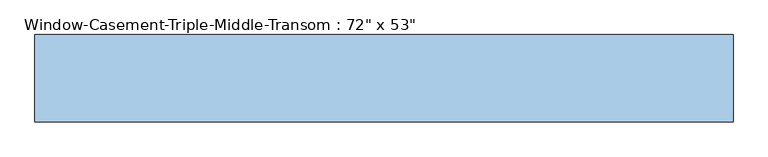
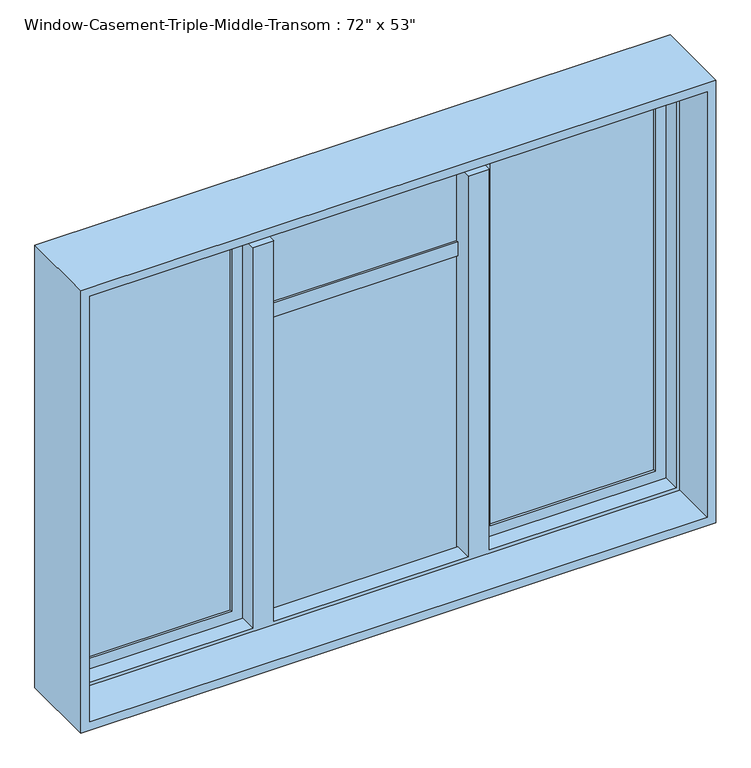
"""IFC4 building model written with IfcOpenShell, lengths in millimetres: window geometry."""

from ifc_helpers import new_model, si_unit, frame, origin, place, context, project, spatial, polyline, outline, extrude, faceted_brep, source, transform, mapped, element, save


def window_7a1f68bc(model_context):
    return source(origin(), model_context, "Body", "SolidModel", [
        extrude(outline(polyline([(2235.2, 330.2), (939.8, 330.2), (939.8, 889.0), (2235.2, 889.0), (2235.2, 330.2)]), holes=[polyline([(2193.3296875, 847.1296875), (981.6703125, 847.1296875), (981.6703125, 372.0703125), (2193.3296875, 372.0703125), (2193.3296875, 847.1296875)])]), frame((0.0, 73.025, 0.0), z_axis=(0.0, 1.0, 0.0), x_axis=(0.0, 0.0, 1.0)), (0.0, 0.0, 1.0), 31.75),
        extrude(outline(polyline([(2235.2, -889.0), (939.8, -889.0), (939.8, -330.2), (2235.2, -330.2), (2235.2, -889.0)]), holes=[polyline([(2193.3296875, -372.0703125), (981.6703125, -372.0703125), (981.6703125, -847.1296875), (2193.3296875, -847.1296875), (2193.3296875, -372.0703125)])]), frame((0.0, 73.025, 0.0), z_axis=(0.0, 1.0, 0.0), x_axis=(0.0, 0.0, 1.0)), (0.0, 0.0, 1.0), 31.75),
        extrude(outline(polyline([(-372.0703125, 98.425), (-372.0703125, 92.075), (-847.1296875, 92.075), (-847.1296875, 98.425), (-372.0703125, 98.425)])), frame((0.0, 0.0, 949.9203125), z_axis=(0.0, 0.0, 1.0), x_axis=(1.0, 0.0, 0.0)), (0.0, 0.0, 1.0), 1275.159375),
        extrude(outline(polyline([(-372.0703125, 85.725), (-372.0703125, 79.375), (-847.1296875, 79.375), (-847.1296875, 85.725), (-372.0703125, 85.725)])), frame((0.0, 0.0, 949.9203125), z_axis=(0.0, 0.0, 1.0), x_axis=(1.0, 0.0, 0.0)), (0.0, 0.0, 1.0), 1275.159375),
        extrude(outline(polyline([(847.1296875, 98.425), (847.1296875, 92.075), (372.0703125, 92.075), (372.0703125, 98.425), (847.1296875, 98.425)])), frame((0.0, 0.0, 949.9203125), z_axis=(0.0, 0.0, 1.0), x_axis=(1.0, 0.0, 0.0)), (0.0, 0.0, 1.0), 1275.159375),
        extrude(outline(polyline([(847.1296875, 85.725), (847.1296875, 79.375), (372.0703125, 79.375), (372.0703125, 85.725), (847.1296875, 85.725)])), frame((0.0, 0.0, 949.9203125), z_axis=(0.0, 0.0, 1.0), x_axis=(1.0, 0.0, 0.0)), (0.0, 0.0, 1.0), 1275.159375),
        extrude(outline(polyline([(279.4, 104.775), (279.4, 73.025), (-279.4, 73.025), (-279.4, 104.775), (279.4, 104.775)])), frame((0.0, 0.0, 1835.8048438), z_axis=(0.0, 0.0, 1.0), x_axis=(1.0, 0.0, 0.0)), (0.0, 0.0, 1.0), 41.8703125),
        extrude(outline(polyline([(279.4, 98.425), (279.4, 92.075), (-279.4, 92.075), (-279.4, 98.425), (279.4, 98.425)])), frame((0.0, 0.0, 939.8), z_axis=(0.0, 0.0, 1.0), x_axis=(1.0, 0.0, 0.0)), (0.0, 0.0, 1.0), 896.0048437),
        extrude(outline(polyline([(279.4, 85.725), (279.4, 79.375), (-279.4, 79.375), (-279.4, 85.725), (279.4, 85.725)])), frame((0.0, 0.0, 939.8), z_axis=(0.0, 0.0, 1.0), x_axis=(1.0, 0.0, 0.0)), (0.0, 0.0, 1.0), 896.0048437),
        extrude(outline(polyline([(279.4, 98.425), (279.4, 92.075), (-279.4, 92.075), (-279.4, 98.425), (279.4, 98.425)])), frame((0.0, 0.0, 1877.6751563), z_axis=(0.0, 0.0, 1.0), x_axis=(1.0, 0.0, 0.0)), (0.0, 0.0, 1.0), 357.5248438),
        extrude(outline(polyline([(279.4, 85.725), (279.4, 79.375), (-279.4, 79.375), (-279.4, 85.725), (279.4, 85.725)])), frame((0.0, 0.0, 1877.6751563), z_axis=(0.0, 0.0, 1.0), x_axis=(1.0, 0.0, 0.0)), (0.0, 0.0, 1.0), 357.5248438),
        faceted_brep([(-889.0, 73.025, 2235.2), (-889.0, 114.3, 2235.2), (889.0, 114.3, 2235.2), (889.0, 73.025, 2235.2), (-878.8796875, 22.225, 2225.0796875), (-878.8796875, 73.025, 2225.0796875), (878.8796875, 73.025, 2225.0796875), (878.8796875, 22.225, 2225.0796875), (-889.0, -114.3, 2235.2), (-889.0, 22.225, 2235.2), (889.0, 22.225, 2235.2), (889.0, -114.3, 2235.2), (-914.4, 114.3, 2260.6), (-914.4, -114.3, 2260.6), (914.4, -114.3, 2260.6), (914.4, 114.3, 2260.6), (889.0, 114.3, 939.8), (889.0, 73.025, 939.8), (878.8796875, 73.025, 949.9203125), (878.8796875, 22.225, 949.9203125), (889.0, 22.225, 939.8), (889.0, -114.3, 939.8), (914.4, -114.3, 914.4), (914.4, 114.3, 914.4), (330.2, 73.025, 939.8), (-889.0, 114.3, 939.8), (-889.0, 73.025, 939.8), (-330.2, 73.025, 939.8), (-330.2, 111.125, 939.8), (-279.4, 111.125, 939.8), (-279.4, 73.025, 939.8), (279.4, 73.025, 939.8), (279.4, 111.125, 939.8), (330.2, 111.125, 939.8), (340.3203125, 73.025, 949.9203125), (340.3203125, 22.225, 949.9203125), (-878.8796875, 73.025, 949.9203125), (-878.8796875, 22.225, 949.9203125), (-340.3203125, 22.225, 949.9203125), (-340.3203125, 73.025, 949.9203125), (279.4, 73.025, 949.9203125), (-279.4, 73.025, 949.9203125), (-279.4, 22.225, 949.9203125), (279.4, 22.225, 949.9203125), (-889.0, 22.225, 939.8), (-889.0, -114.3, 939.8), (-914.4, -114.3, 914.4), (-914.4, 114.3, 914.4), (330.2, 73.025, 2108.2), (340.3203125, 73.025, 2108.2), (-340.3203125, 73.025, 2108.2), (-330.2, 73.025, 2108.2), (-279.4, 111.125, 2108.2), (-330.2, 111.125, 2108.2), (-340.3203125, 22.225, 2108.2), (-279.4, 22.225, 2108.2), (330.2, 111.125, 2108.2), (279.4, 111.125, 2108.2), (279.4, 22.225, 2108.2), (340.3203125, 22.225, 2108.2)], [[[0, 1, 2, 3]], [[4, 5, 6, 7]], [[8, 9, 10, 11]], [[12, 13, 14, 15]], [[3, 2, 16, 17]], [[7, 6, 18, 19]], [[11, 10, 20, 21]], [[15, 14, 22, 23]], [[24, 17, 16, 25, 26, 27, 28, 29, 30, 31, 32, 33]], [[19, 18, 34, 35]], [[36, 37, 38, 39]], [[40, 41, 42, 43]], [[21, 20, 44, 45]], [[23, 22, 46, 47]], [[1, 0, 26, 25]], [[0, 3, 17, 24, 48, 49, 34, 18, 6, 5, 36, 39, 50, 51, 27, 26]], [[41, 40, 31, 30]], [[5, 4, 37, 36]], [[9, 8, 45, 44]], [[14, 13, 46, 22], [8, 11, 21, 45]], [[13, 12, 47, 46]], [[12, 15, 23, 47], [2, 1, 25, 16]], [[52, 53, 51, 50, 54, 55]], [[56, 57, 58, 59, 49, 48]], [[53, 52, 29, 28]], [[27, 51, 53, 28]], [[52, 55, 42, 41, 30, 29]], [[57, 56, 33, 32]], [[58, 57, 32, 31, 40, 43]], [[56, 48, 24, 33]], [[54, 50, 39, 38]], [[49, 59, 35, 34]], [[10, 9, 44, 20], [4, 7, 19, 35, 59, 58, 43, 42, 55, 54, 38, 37]]]),
    ])


if __name__ == "__main__":
    model = new_model("IFC4")
    model_context = context("Model", 3, world=origin())
    ifc_project = project(units=[si_unit("LENGTHUNIT", "METRE", prefix="MILLI")], contexts=[model_context])
    site = spatial("IfcSite", under=ifc_project)
    building = spatial("IfcBuilding", under=site)
    placement = place(None, origin())
    window_shape = window_7a1f68bc(model_context)
    element("IfcWindow", 1, ObjectType="Window-Casement-Triple-Middle-Transom : 72\" x 53\"", at=placement, inside=building, context=model_context, shape_type="MappedRepresentation", body=[
        mapped(window_shape, transform((0.0, 0.0, 0.0), x_axis=(1.0, 0.0, 0.0), y_axis=(0.0, 1.0, 0.0), z_axis=(0.0, 0.0, 1.0))),
    ])
    save(model, "model.ifc")

# Revit data of these elements
# Type "Window-Casement-Triple-Middle-Transom : 72\" x 53\""
#   Type Mark = "52"
#   Fire Rating = "0.5h"
#   Assembly Code = "B2020100"
#   Analytic Construction = "Double glazing - domestic"
#   Window Width = 2' - 0"
#   Window Inset [instance default] = 0' - 0 5/8"
#   Wall Thickness [instance default] = 0' - 6"
#   Visual Light Transmittance = 0.81
#   Transom Height Ratio = 0.3
#   Thermal Resistance (R) = 0.319569 (m²·K)/W
#   Solar Heat Gain Coefficient = 0.76
#   Rough Width = 6' - 0 1/2"
#   Rough Height = 4' - 5 1/2"
#   Heat Transfer Coefficient (U) = 3.12929 W/(m²·K)
#   Height = 4' - 5"
#   Transom Height = 1' - 3.9"
#   Frame Gap 3 [instance default] = 0' - 1 83/128"
#   Frame Gap 2 [instance default] = 0' - 0 5/8"
#   Frame Gap 1 = 0' - 1 51/128"
#   Default Sill Height = 3' - 0"
#   Width = 6' - 0"
#   Frame Material = Metal - Aluminum
#   Glass Panel Material = Glass
#   Wall Closure = (empty or 0)
# Element 1 (IfcWindow, "Window-Casement-Triple-Middle-Transom : 72\" x 53\"")
#   Wall Thickness = 0' - 9"
#   Materials on its faces: "Metal - Aluminum", "Glass"
# Materials
#   "Metal - Aluminum": class "Metal", colour RGB 247 247 247, transparency 0
#   "Glass": class "Glass", colour RGB 0 128 192, transparency 0.9, Description = "Soda Lime Glass", Cost = 0
